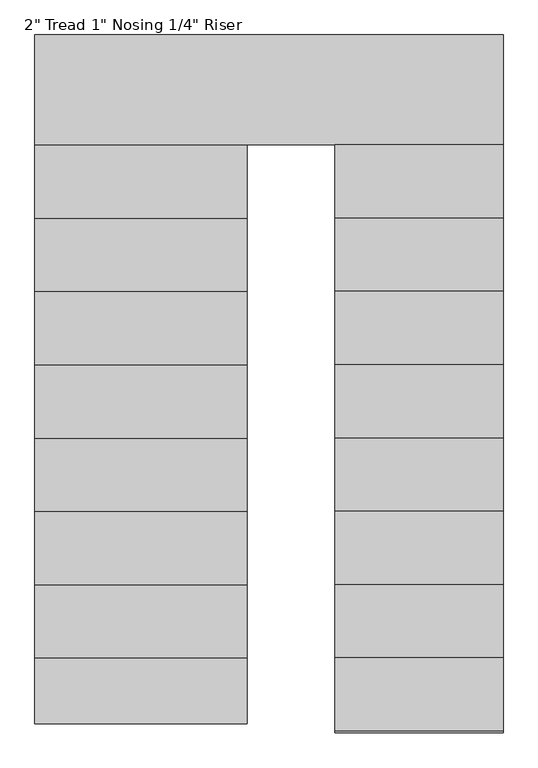
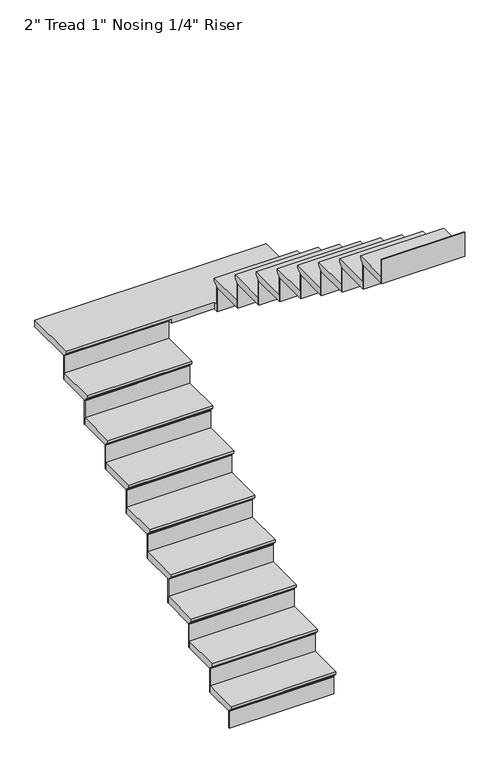
"""IFC4 building model written with IfcOpenShell, lengths in millimetres: stair flight geometry."""

from ifc_helpers import new_model, si_unit, origin, place, context, project, spatial, faceted_brep, source, transform, mapped, element, save


def stair_flight_e23070b7(model_context):
    return source(origin(), model_context, "Body", "Brep", [
        faceted_brep([(3394.0891134, -7650.9822004, 6559.55), (3394.0891134, -7650.9822004, 6578.6), (2657.4891134, -7650.9822004, 6578.6), (2657.4891134, -7650.9822004, 6559.55), (3394.0891134, -7625.5822004, 6534.15), (2657.4891134, -7625.5822004, 6534.15), (3394.0891134, -7396.9822004, 6578.6), (2657.4891134, -7396.9822004, 6578.6), (2657.4891134, -7625.5822004, 6527.8), (2657.4891134, -7396.9822004, 6527.8), (3394.0891134, -7396.9822004, 6527.8), (3394.0891134, -7625.5822004, 6527.8)], [[[0, 1, 2, 3]], [[4, 0, 3, 5]], [[2, 1, 6, 7]], [[8, 9, 10, 11]], [[2, 7, 9, 8, 5, 3]], [[8, 11, 4, 5]], [[6, 1, 0, 4, 11, 10]], [[7, 6, 10, 9]]]),
        faceted_brep([(3394.0891134, -7625.5822004, 6527.8), (3394.0891134, -7625.5822004, 6400.8), (3394.0891134, -7619.2322004, 6400.8), (3394.0891134, -7619.2322004, 6527.8), (2657.4891134, -7625.5822004, 6527.8), (2657.4891134, -7619.2322004, 6527.8), (2657.4891134, -7619.2322004, 6400.8), (2657.4891134, -7625.5822004, 6400.8)], [[[0, 1, 2, 3]], [[4, 5, 6, 7]], [[1, 0, 4, 7]], [[2, 1, 7, 6]], [[3, 2, 6, 5]], [[0, 3, 5, 4]]]),
        faceted_brep([(3394.0891134, -7396.9822004, 6705.6), (3394.0891134, -7396.9822004, 6527.8), (3394.0891134, -7390.6322004, 6527.8), (3394.0891134, -7390.6322004, 6705.6), (2657.4891134, -7396.9822004, 6705.6), (2657.4891134, -7390.6322004, 6705.6), (2657.4891134, -7390.6322004, 6527.8), (2657.4891134, -7396.9822004, 6527.8)], [[[0, 1, 2, 3]], [[4, 5, 6, 7]], [[1, 0, 4, 7]], [[2, 1, 7, 6]], [[3, 2, 6, 5]], [[0, 3, 5, 4]]]),
        faceted_brep([(2657.4891134, -7422.3822004, 6756.4), (3394.0891134, -7422.3822004, 6756.4), (3394.0891134, -7142.9822004, 6756.4), (2657.4891134, -7142.9822004, 6756.4), (2657.4891134, -7396.9822004, 6705.6), (2657.4891134, -7142.9822004, 6705.6), (3394.0891134, -7142.9822004, 6705.6), (3394.0891134, -7396.9822004, 6705.6), (2657.4891134, -7396.9822004, 6711.95), (2657.4891134, -7422.3822004, 6737.35), (3394.0891134, -7396.9822004, 6711.95), (3394.0891134, -7422.3822004, 6737.35)], [[[0, 1, 2, 3]], [[4, 5, 6, 7]], [[0, 3, 5, 4, 8, 9]], [[4, 7, 10, 8]], [[2, 1, 11, 10, 7, 6]], [[3, 2, 6, 5]], [[11, 1, 0, 9]], [[10, 11, 9, 8]]]),
        faceted_brep([(3394.0891134, -7142.9822004, 6883.4), (3394.0891134, -7142.9822004, 6705.6), (3394.0891134, -7136.6322004, 6705.6), (3394.0891134, -7136.6322004, 6883.4), (2657.4891134, -7142.9822004, 6883.4), (2657.4891134, -7136.6322004, 6883.4), (2657.4891134, -7136.6322004, 6705.6), (2657.4891134, -7142.9822004, 6705.6)], [[[0, 1, 2, 3]], [[4, 5, 6, 7]], [[1, 0, 4, 7]], [[2, 1, 7, 6]], [[3, 2, 6, 5]], [[0, 3, 5, 4]]]),
        faceted_brep([(2657.4891134, -7168.3822004, 6934.2), (3394.0891134, -7168.3822004, 6934.2), (3394.0891134, -6888.9822004, 6934.2), (2657.4891134, -6888.9822004, 6934.2), (2657.4891134, -7142.9822004, 6883.4), (2657.4891134, -6888.9822004, 6883.4), (3394.0891134, -6888.9822004, 6883.4), (3394.0891134, -7142.9822004, 6883.4), (2657.4891134, -7142.9822004, 6889.75), (2657.4891134, -7168.3822004, 6915.15), (3394.0891134, -7142.9822004, 6889.75), (3394.0891134, -7168.3822004, 6915.15)], [[[0, 1, 2, 3]], [[4, 5, 6, 7]], [[0, 3, 5, 4, 8, 9]], [[4, 7, 10, 8]], [[2, 1, 11, 10, 7, 6]], [[3, 2, 6, 5]], [[11, 1, 0, 9]], [[10, 11, 9, 8]]]),
        faceted_brep([(3394.0891134, -6888.9822004, 7061.2), (3394.0891134, -6888.9822004, 6883.4), (3394.0891134, -6882.6322004, 6883.4), (3394.0891134, -6882.6322004, 7061.2), (2657.4891134, -6888.9822004, 7061.2), (2657.4891134, -6882.6322004, 7061.2), (2657.4891134, -6882.6322004, 6883.4), (2657.4891134, -6888.9822004, 6883.4)], [[[0, 1, 2, 3]], [[4, 5, 6, 7]], [[1, 0, 4, 7]], [[2, 1, 7, 6]], [[3, 2, 6, 5]], [[0, 3, 5, 4]]]),
        faceted_brep([(2657.4891134, -6914.3822004, 7112.0), (3394.0891134, -6914.3822004, 7112.0), (3394.0891134, -6634.9822004, 7112.0), (2657.4891134, -6634.9822004, 7112.0), (2657.4891134, -6888.9822004, 7061.2), (2657.4891134, -6634.9822004, 7061.2), (3394.0891134, -6634.9822004, 7061.2), (3394.0891134, -6888.9822004, 7061.2), (2657.4891134, -6888.9822004, 7067.55), (2657.4891134, -6914.3822004, 7092.95), (3394.0891134, -6888.9822004, 7067.55), (3394.0891134, -6914.3822004, 7092.95)], [[[0, 1, 2, 3]], [[4, 5, 6, 7]], [[0, 3, 5, 4, 8, 9]], [[4, 7, 10, 8]], [[2, 1, 11, 10, 7, 6]], [[3, 2, 6, 5]], [[11, 1, 0, 9]], [[10, 11, 9, 8]]]),
        faceted_brep([(3394.0891134, -6634.9822004, 7239.0), (3394.0891134, -6634.9822004, 7061.2), (3394.0891134, -6628.6322004, 7061.2), (3394.0891134, -6628.6322004, 7239.0), (2657.4891134, -6634.9822004, 7239.0), (2657.4891134, -6628.6322004, 7239.0), (2657.4891134, -6628.6322004, 7061.2), (2657.4891134, -6634.9822004, 7061.2)], [[[0, 1, 2, 3]], [[4, 5, 6, 7]], [[1, 0, 4, 7]], [[2, 1, 7, 6]], [[3, 2, 6, 5]], [[0, 3, 5, 4]]]),
        faceted_brep([(2657.4891134, -6660.3822004, 7289.8), (3394.0891134, -6660.3822004, 7289.8), (3394.0891134, -6380.9822004, 7289.8), (2657.4891134, -6380.9822004, 7289.8), (2657.4891134, -6634.9822004, 7239.0), (2657.4891134, -6380.9822004, 7239.0), (3394.0891134, -6380.9822004, 7239.0), (3394.0891134, -6634.9822004, 7239.0), (2657.4891134, -6634.9822004, 7245.35), (2657.4891134, -6660.3822004, 7270.75), (3394.0891134, -6634.9822004, 7245.35), (3394.0891134, -6660.3822004, 7270.75)], [[[0, 1, 2, 3]], [[4, 5, 6, 7]], [[0, 3, 5, 4, 8, 9]], [[4, 7, 10, 8]], [[2, 1, 11, 10, 7, 6]], [[3, 2, 6, 5]], [[11, 1, 0, 9]], [[10, 11, 9, 8]]]),
        faceted_brep([(3394.0891134, -6380.9822004, 7416.8), (3394.0891134, -6380.9822004, 7239.0), (3394.0891134, -6374.6322004, 7239.0), (3394.0891134, -6374.6322004, 7416.8), (2657.4891134, -6380.9822004, 7416.8), (2657.4891134, -6374.6322004, 7416.8), (2657.4891134, -6374.6322004, 7239.0), (2657.4891134, -6380.9822004, 7239.0)], [[[0, 1, 2, 3]], [[4, 5, 6, 7]], [[1, 0, 4, 7]], [[2, 1, 7, 6]], [[3, 2, 6, 5]], [[0, 3, 5, 4]]]),
        faceted_brep([(2657.4891134, -6406.3822004, 7467.6), (3394.0891134, -6406.3822004, 7467.6), (3394.0891134, -6126.9822004, 7467.6), (2657.4891134, -6126.9822004, 7467.6), (2657.4891134, -6380.9822004, 7416.8), (2657.4891134, -6126.9822004, 7416.8), (3394.0891134, -6126.9822004, 7416.8), (3394.0891134, -6380.9822004, 7416.8), (2657.4891134, -6380.9822004, 7423.15), (2657.4891134, -6406.3822004, 7448.55), (3394.0891134, -6380.9822004, 7423.15), (3394.0891134, -6406.3822004, 7448.55)], [[[0, 1, 2, 3]], [[4, 5, 6, 7]], [[0, 3, 5, 4, 8, 9]], [[4, 7, 10, 8]], [[2, 1, 11, 10, 7, 6]], [[3, 2, 6, 5]], [[11, 1, 0, 9]], [[10, 11, 9, 8]]]),
        faceted_brep([(3394.0891134, -6126.9822004, 7594.6), (3394.0891134, -6126.9822004, 7416.8), (3394.0891134, -6120.6322004, 7416.8), (3394.0891134, -6120.6322004, 7594.6), (2657.4891134, -6126.9822004, 7594.6), (2657.4891134, -6120.6322004, 7594.6), (2657.4891134, -6120.6322004, 7416.8), (2657.4891134, -6126.9822004, 7416.8)], [[[0, 1, 2, 3]], [[4, 5, 6, 7]], [[1, 0, 4, 7]], [[2, 1, 7, 6]], [[3, 2, 6, 5]], [[0, 3, 5, 4]]]),
        faceted_brep([(2657.4891134, -6152.3822004, 7645.4), (3394.0891134, -6152.3822004, 7645.4), (3394.0891134, -5872.9822004, 7645.4), (2657.4891134, -5872.9822004, 7645.4), (2657.4891134, -6126.9822004, 7594.6), (2657.4891134, -5872.9822004, 7594.6), (3394.0891134, -5872.9822004, 7594.6), (3394.0891134, -6126.9822004, 7594.6), (2657.4891134, -6126.9822004, 7600.95), (2657.4891134, -6152.3822004, 7626.35), (3394.0891134, -6126.9822004, 7600.95), (3394.0891134, -6152.3822004, 7626.35)], [[[0, 1, 2, 3]], [[4, 5, 6, 7]], [[0, 3, 5, 4, 8, 9]], [[4, 7, 10, 8]], [[2, 1, 11, 10, 7, 6]], [[3, 2, 6, 5]], [[11, 1, 0, 9]], [[10, 11, 9, 8]]]),
        faceted_brep([(3394.0891134, -5872.9822004, 7772.4), (3394.0891134, -5872.9822004, 7594.6), (3394.0891134, -5866.6322004, 7594.6), (3394.0891134, -5866.6322004, 7772.4), (2657.4891134, -5872.9822004, 7772.4), (2657.4891134, -5866.6322004, 7772.4), (2657.4891134, -5866.6322004, 7594.6), (2657.4891134, -5872.9822004, 7594.6)], [[[0, 1, 2, 3]], [[4, 5, 6, 7]], [[1, 0, 4, 7]], [[2, 1, 7, 6]], [[3, 2, 6, 5]], [[0, 3, 5, 4]]]),
        faceted_brep([(2657.4891134, -5898.3822004, 7823.2), (3394.0891134, -5898.3822004, 7823.2), (3394.0891134, -5618.9822004, 7823.2), (2657.4891134, -5618.9822004, 7823.2), (2657.4891134, -5872.9822004, 7772.4), (2657.4891134, -5618.9822004, 7772.4), (3394.0891134, -5618.9822004, 7772.4), (3394.0891134, -5872.9822004, 7772.4), (2657.4891134, -5872.9822004, 7778.75), (2657.4891134, -5898.3822004, 7804.15), (3394.0891134, -5872.9822004, 7778.75), (3394.0891134, -5898.3822004, 7804.15)], [[[0, 1, 2, 3]], [[4, 5, 6, 7]], [[0, 3, 5, 4, 8, 9]], [[4, 7, 10, 8]], [[2, 1, 11, 10, 7, 6]], [[3, 2, 6, 5]], [[11, 1, 0, 9]], [[10, 11, 9, 8]]]),
        faceted_brep([(3394.0891134, -5618.9822004, 7950.2), (3394.0891134, -5618.9822004, 7772.4), (3394.0891134, -5612.6322004, 7772.4), (3394.0891134, -5612.6322004, 7950.2), (2657.4891134, -5618.9822004, 7950.2), (2657.4891134, -5612.6322004, 7950.2), (2657.4891134, -5612.6322004, 7772.4), (2657.4891134, -5618.9822004, 7772.4)], [[[0, 1, 2, 3]], [[4, 5, 6, 7]], [[1, 0, 4, 7]], [[2, 1, 7, 6]], [[3, 2, 6, 5]], [[0, 3, 5, 4]]]),
        faceted_brep([(4281.7311655, -5669.7822004, 8001.0), (4281.7311655, -5263.3822004, 8001.0), (2657.4891134, -5263.3822004, 8001.0), (2657.4891134, -5644.3822004, 8001.0), (3698.8891134, -5644.3822004, 8001.0), (3698.8891134, -5669.7822004, 8001.0), (4281.7311655, -5263.3822004, 7950.2), (4281.7311655, -5669.7822004, 7950.2), (3698.8891134, -5669.7822004, 7950.2), (3698.8891134, -5644.3822004, 7950.2), (3394.0891134, -5644.3822004, 7950.2), (3394.0891134, -5618.9822004, 7950.2), (2657.4891134, -5618.9822004, 7950.2), (2657.4891134, -5263.3822004, 7950.2), (3394.0891134, -5618.9822004, 7956.55), (2657.4891134, -5618.9822004, 7956.55), (2657.4891134, -5644.3822004, 7981.95), (3394.0891134, -5644.3822004, 7981.95)], [[[0, 1, 2, 3, 4, 5]], [[6, 7, 8, 9, 10, 11, 12, 13]], [[1, 0, 7, 6]], [[2, 1, 6, 13]], [[12, 11, 14, 15]], [[4, 3, 16, 17, 10, 9]], [[5, 4, 9, 8]], [[0, 5, 8, 7]], [[16, 15, 14, 17]], [[3, 2, 13, 12, 15, 16]], [[11, 10, 17, 14]]]),
        faceted_brep([(3698.8891134, -5669.7822004, 8128.0), (3698.8891134, -5669.7822004, 7950.2), (3698.8891134, -5676.1322004, 7950.2), (3698.8891134, -5676.1322004, 8128.0), (4281.7311655, -5669.7822004, 8128.0), (4281.7311655, -5676.1322004, 8128.0), (4281.7311655, -5676.1322004, 7950.2), (4281.7311655, -5669.7822004, 7950.2)], [[[0, 1, 2, 3]], [[4, 5, 6, 7]], [[1, 0, 4, 7]], [[2, 1, 7, 6]], [[3, 2, 6, 5]], [[0, 3, 5, 4]]]),
        faceted_brep([(4281.7311655, -5644.3822004, 8178.8), (3698.8891134, -5644.3822004, 8178.8), (3698.8891134, -5923.7822004, 8178.8), (4281.7311655, -5923.7822004, 8178.8), (4281.7311655, -5669.7822004, 8128.0), (4281.7311655, -5923.7822004, 8128.0), (3698.8891134, -5923.7822004, 8128.0), (3698.8891134, -5669.7822004, 8128.0), (4281.7311655, -5669.7822004, 8134.35), (4281.7311655, -5644.3822004, 8159.75), (3698.8891134, -5669.7822004, 8134.35), (3698.8891134, -5644.3822004, 8159.75)], [[[0, 1, 2, 3]], [[4, 5, 6, 7]], [[0, 3, 5, 4, 8, 9]], [[4, 7, 10, 8]], [[2, 1, 11, 10, 7, 6]], [[3, 2, 6, 5]], [[11, 1, 0, 9]], [[10, 11, 9, 8]]]),
        faceted_brep([(3698.8891134, -5923.7822004, 8305.8), (3698.8891134, -5923.7822004, 8128.0), (3698.8891134, -5930.1322004, 8128.0), (3698.8891134, -5930.1322004, 8305.8), (4281.7311655, -5923.7822004, 8305.8), (4281.7311655, -5930.1322004, 8305.8), (4281.7311655, -5930.1322004, 8128.0), (4281.7311655, -5923.7822004, 8128.0)], [[[0, 1, 2, 3]], [[4, 5, 6, 7]], [[1, 0, 4, 7]], [[2, 1, 7, 6]], [[3, 2, 6, 5]], [[0, 3, 5, 4]]]),
        faceted_brep([(4281.7311655, -5898.3822004, 8356.6), (3698.8891134, -5898.3822004, 8356.6), (3698.8891134, -6177.7822004, 8356.6), (4281.7311655, -6177.7822004, 8356.6), (4281.7311655, -5923.7822004, 8305.8), (4281.7311655, -6177.7822004, 8305.8), (3698.8891134, -6177.7822004, 8305.8), (3698.8891134, -5923.7822004, 8305.8), (4281.7311655, -5923.7822004, 8312.15), (4281.7311655, -5898.3822004, 8337.55), (3698.8891134, -5923.7822004, 8312.15), (3698.8891134, -5898.3822004, 8337.55)], [[[0, 1, 2, 3]], [[4, 5, 6, 7]], [[0, 3, 5, 4, 8, 9]], [[4, 7, 10, 8]], [[2, 1, 11, 10, 7, 6]], [[3, 2, 6, 5]], [[11, 1, 0, 9]], [[10, 11, 9, 8]]]),
        faceted_brep([(3698.8891134, -6177.7822004, 8483.6), (3698.8891134, -6177.7822004, 8305.8), (3698.8891134, -6184.1322004, 8305.8), (3698.8891134, -6184.1322004, 8483.6), (4281.7311655, -6177.7822004, 8483.6), (4281.7311655, -6184.1322004, 8483.6), (4281.7311655, -6184.1322004, 8305.8), (4281.7311655, -6177.7822004, 8305.8)], [[[0, 1, 2, 3]], [[4, 5, 6, 7]], [[1, 0, 4, 7]], [[2, 1, 7, 6]], [[3, 2, 6, 5]], [[0, 3, 5, 4]]]),
        faceted_brep([(4281.7311655, -6152.3822004, 8534.4), (3698.8891134, -6152.3822004, 8534.4), (3698.8891134, -6431.7822004, 8534.4), (4281.7311655, -6431.7822004, 8534.4), (4281.7311655, -6177.7822004, 8483.6), (4281.7311655, -6431.7822004, 8483.6), (3698.8891134, -6431.7822004, 8483.6), (3698.8891134, -6177.7822004, 8483.6), (4281.7311655, -6177.7822004, 8489.95), (4281.7311655, -6152.3822004, 8515.35), (3698.8891134, -6177.7822004, 8489.95), (3698.8891134, -6152.3822004, 8515.35)], [[[0, 1, 2, 3]], [[4, 5, 6, 7]], [[0, 3, 5, 4, 8, 9]], [[4, 7, 10, 8]], [[2, 1, 11, 10, 7, 6]], [[3, 2, 6, 5]], [[11, 1, 0, 9]], [[10, 11, 9, 8]]]),
        faceted_brep([(3698.8891134, -6431.7822004, 8661.4), (3698.8891134, -6431.7822004, 8483.6), (3698.8891134, -6438.1322004, 8483.6), (3698.8891134, -6438.1322004, 8661.4), (4281.7311655, -6431.7822004, 8661.4), (4281.7311655, -6438.1322004, 8661.4), (4281.7311655, -6438.1322004, 8483.6), (4281.7311655, -6431.7822004, 8483.6)], [[[0, 1, 2, 3]], [[4, 5, 6, 7]], [[1, 0, 4, 7]], [[2, 1, 7, 6]], [[3, 2, 6, 5]], [[0, 3, 5, 4]]]),
        faceted_brep([(4281.7311655, -6406.3822004, 8712.2), (3698.8891134, -6406.3822004, 8712.2), (3698.8891134, -6685.7822004, 8712.2), (4281.7311655, -6685.7822004, 8712.2), (4281.7311655, -6431.7822004, 8661.4), (4281.7311655, -6685.7822004, 8661.4), (3698.8891134, -6685.7822004, 8661.4), (3698.8891134, -6431.7822004, 8661.4), (4281.7311655, -6431.7822004, 8667.75), (4281.7311655, -6406.3822004, 8693.15), (3698.8891134, -6431.7822004, 8667.75), (3698.8891134, -6406.3822004, 8693.15)], [[[0, 1, 2, 3]], [[4, 5, 6, 7]], [[0, 3, 5, 4, 8, 9]], [[4, 7, 10, 8]], [[2, 1, 11, 10, 7, 6]], [[3, 2, 6, 5]], [[11, 1, 0, 9]], [[10, 11, 9, 8]]]),
        faceted_brep([(3698.8891134, -6685.7822004, 8839.2), (3698.8891134, -6685.7822004, 8661.4), (3698.8891134, -6692.1322004, 8661.4), (3698.8891134, -6692.1322004, 8839.2), (4281.7311655, -6685.7822004, 8839.2), (4281.7311655, -6692.1322004, 8839.2), (4281.7311655, -6692.1322004, 8661.4), (4281.7311655, -6685.7822004, 8661.4)], [[[0, 1, 2, 3]], [[4, 5, 6, 7]], [[1, 0, 4, 7]], [[2, 1, 7, 6]], [[3, 2, 6, 5]], [[0, 3, 5, 4]]]),
        faceted_brep([(4281.7311655, -6660.3822004, 8890.0), (3698.8891134, -6660.3822004, 8890.0), (3698.8891134, -6939.7822004, 8890.0), (4281.7311655, -6939.7822004, 8890.0), (4281.7311655, -6685.7822004, 8839.2), (4281.7311655, -6939.7822004, 8839.2), (3698.8891134, -6939.7822004, 8839.2), (3698.8891134, -6685.7822004, 8839.2), (4281.7311655, -6685.7822004, 8845.55), (4281.7311655, -6660.3822004, 8870.95), (3698.8891134, -6685.7822004, 8845.55), (3698.8891134, -6660.3822004, 8870.95)], [[[0, 1, 2, 3]], [[4, 5, 6, 7]], [[0, 3, 5, 4, 8, 9]], [[4, 7, 10, 8]], [[2, 1, 11, 10, 7, 6]], [[3, 2, 6, 5]], [[11, 1, 0, 9]], [[10, 11, 9, 8]]]),
        faceted_brep([(3698.8891134, -6939.7822004, 9017.0), (3698.8891134, -6939.7822004, 8839.2), (3698.8891134, -6946.1322004, 8839.2), (3698.8891134, -6946.1322004, 9017.0), (4281.7311655, -6939.7822004, 9017.0), (4281.7311655, -6946.1322004, 9017.0), (4281.7311655, -6946.1322004, 8839.2), (4281.7311655, -6939.7822004, 8839.2)], [[[0, 1, 2, 3]], [[4, 5, 6, 7]], [[1, 0, 4, 7]], [[2, 1, 7, 6]], [[3, 2, 6, 5]], [[0, 3, 5, 4]]]),
        faceted_brep([(4281.7311655, -6914.3822004, 9067.8), (3698.8891134, -6914.3822004, 9067.8), (3698.8891134, -7193.7822004, 9067.8), (4281.7311655, -7193.7822004, 9067.8), (4281.7311655, -6939.7822004, 9017.0), (4281.7311655, -7193.7822004, 9017.0), (3698.8891134, -7193.7822004, 9017.0), (3698.8891134, -6939.7822004, 9017.0), (4281.7311655, -6939.7822004, 9023.35), (4281.7311655, -6914.3822004, 9048.75), (3698.8891134, -6939.7822004, 9023.35), (3698.8891134, -6914.3822004, 9048.75)], [[[0, 1, 2, 3]], [[4, 5, 6, 7]], [[0, 3, 5, 4, 8, 9]], [[4, 7, 10, 8]], [[2, 1, 11, 10, 7, 6]], [[3, 2, 6, 5]], [[11, 1, 0, 9]], [[10, 11, 9, 8]]]),
        faceted_brep([(3698.8891134, -7193.7822004, 9194.8), (3698.8891134, -7193.7822004, 9017.0), (3698.8891134, -7200.1322004, 9017.0), (3698.8891134, -7200.1322004, 9194.8), (4281.7311655, -7193.7822004, 9194.8), (4281.7311655, -7200.1322004, 9194.8), (4281.7311655, -7200.1322004, 9017.0), (4281.7311655, -7193.7822004, 9017.0)], [[[0, 1, 2, 3]], [[4, 5, 6, 7]], [[1, 0, 4, 7]], [[2, 1, 7, 6]], [[3, 2, 6, 5]], [[0, 3, 5, 4]]]),
        faceted_brep([(4281.7311655, -7168.3822004, 9245.6), (3698.8891134, -7168.3822004, 9245.6), (3698.8891134, -7447.7822004, 9245.6), (4281.7311655, -7447.7822004, 9245.6), (4281.7311655, -7193.7822004, 9194.8), (4281.7311655, -7447.7822004, 9194.8), (3698.8891134, -7447.7822004, 9194.8), (3698.8891134, -7193.7822004, 9194.8), (4281.7311655, -7193.7822004, 9201.15), (4281.7311655, -7168.3822004, 9226.55), (3698.8891134, -7193.7822004, 9201.15), (3698.8891134, -7168.3822004, 9226.55)], [[[0, 1, 2, 3]], [[4, 5, 6, 7]], [[0, 3, 5, 4, 8, 9]], [[4, 7, 10, 8]], [[2, 1, 11, 10, 7, 6]], [[3, 2, 6, 5]], [[11, 1, 0, 9]], [[10, 11, 9, 8]]]),
        faceted_brep([(3698.8891134, -7447.7822004, 9372.6), (3698.8891134, -7447.7822004, 9194.8), (3698.8891134, -7454.1322004, 9194.8), (3698.8891134, -7454.1322004, 9372.6), (4281.7311655, -7447.7822004, 9372.6), (4281.7311655, -7454.1322004, 9372.6), (4281.7311655, -7454.1322004, 9194.8), (4281.7311655, -7447.7822004, 9194.8)], [[[0, 1, 2, 3]], [[4, 5, 6, 7]], [[1, 0, 4, 7]], [[2, 1, 7, 6]], [[3, 2, 6, 5]], [[0, 3, 5, 4]]]),
        faceted_brep([(3698.8891134, -7676.3822004, 9550.4), (3698.8891134, -7676.3822004, 9372.6), (3698.8891134, -7682.7322004, 9372.6), (3698.8891134, -7682.7322004, 9550.4), (4281.7311655, -7676.3822004, 9550.4), (4281.7311655, -7682.7322004, 9550.4), (4281.7311655, -7682.7322004, 9372.6), (4281.7311655, -7676.3822004, 9372.6)], [[[0, 1, 2, 3]], [[4, 5, 6, 7]], [[1, 0, 4, 7]], [[2, 1, 7, 6]], [[3, 2, 6, 5]], [[0, 3, 5, 4]]]),
        faceted_brep([(4281.7311655, -7422.3822004, 9423.4), (3698.8891134, -7422.3822004, 9423.4), (3698.8891134, -7676.3822004, 9423.4), (4281.7311655, -7676.3822004, 9423.4), (4281.7311655, -7447.7822004, 9372.6), (4281.7311655, -7676.3822004, 9372.6), (3698.8891134, -7676.3822004, 9372.6), (3698.8891134, -7447.7822004, 9372.6), (4281.7311655, -7447.7822004, 9378.95), (4281.7311655, -7422.3822004, 9404.35), (3698.8891134, -7447.7822004, 9378.95), (3698.8891134, -7422.3822004, 9404.35)], [[[0, 1, 2, 3]], [[4, 5, 6, 7]], [[0, 3, 5, 4, 8, 9]], [[4, 7, 10, 8]], [[2, 1, 11, 10, 7, 6]], [[3, 2, 6, 5]], [[11, 1, 0, 9]], [[10, 11, 9, 8]]]),
    ])


if __name__ == "__main__":
    model = new_model("IFC4")
    model_context = context("Model", 3, world=origin())
    ifc_project = project(units=[si_unit("LENGTHUNIT", "METRE", prefix="MILLI")], contexts=[model_context])
    site = spatial("IfcSite", under=ifc_project)
    building = spatial("IfcBuilding", under=site)
    placement = place(None, origin())
    stair_flight_shape = stair_flight_e23070b7(model_context)
    element("IfcStairFlight", 1, ObjectType="2\" Tread 1\" Nosing 1/4\" Riser", at=placement, inside=building, context=model_context, shape_type="MappedRepresentation", body=[
        mapped(stair_flight_shape, transform((0.0, 0.0, 0.0), x_axis=(1.0, 0.0, 0.0), y_axis=(0.0, 1.0, 0.0), z_axis=(0.0, 0.0, 1.0))),
    ])
    save(model, "model.ifc")
